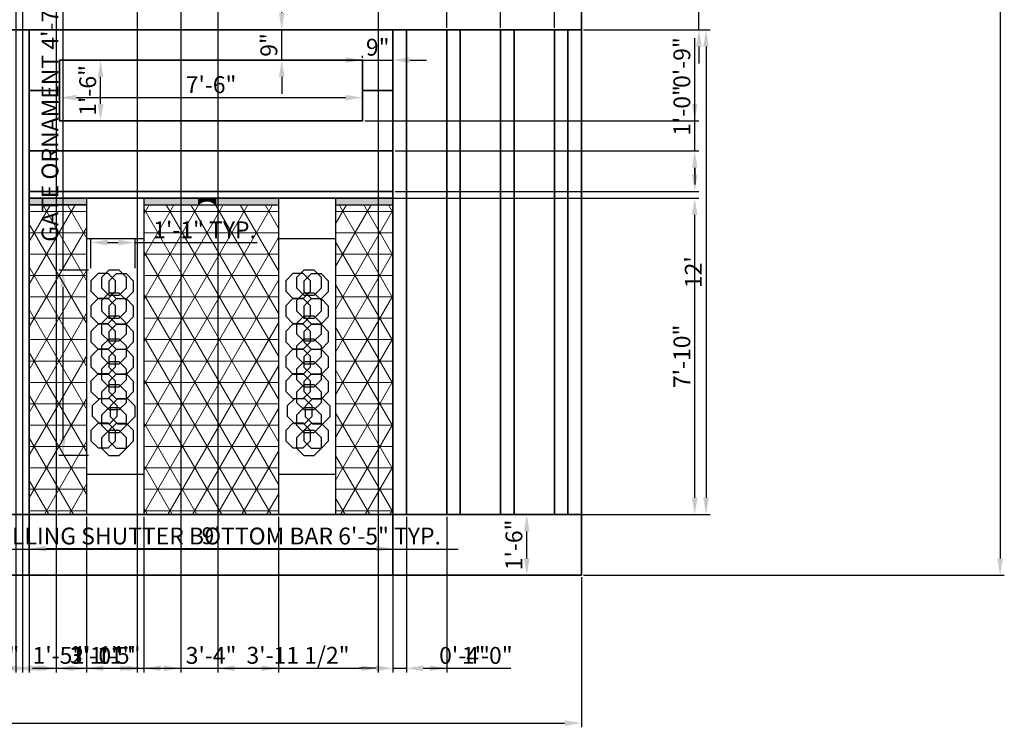
# Model space of a CAD drawing. Units: inches. Extents: x 2406 to 2953, y 1777 to 2285.
# Tile 3 of 5: x 2661 to 2953, y 1777 to 1987. Entities that reach past the tile are written whole.
import ezdxf

# ---------------------------------------------------------------- set-up
doc = ezdxf.new("R2010")
doc.units = ezdxf.units.IN
for name, color, linetype, lineweight in [('A-ANNO-DIMS', 2, 'Continuous', 18), ('A-DOOR', 3, 'Continuous', 25), ('A-ELEV', 7, 'Continuous', 35), ('A-ELEV-PATT', 253, 'Continuous', 13)]:
    doc.layers.add(name, color=color, linetype=linetype, lineweight=lineweight)
doc.styles.get("Standard").update_dxf_attribs({"font": 'arial.ttf'})
doc.dimstyles.new('ISO-25', dxfattribs={"dimtxt": 5, "dimasz": 5, "dimexe": 1.25, "dimexo": 0.625, "dimtad": 1, "dimdec": 0, "dimlunit": 3, "dimtxsty": 'Standard', "dimcen": 2.5, "dimadec": 0, "dimazin": 0, "dimtfac": 1, "dimtdec": 0, "dimtmove": 0, "dimatfit": 3, "dimfxl": 1, "dimarcsym": 0})

# ---------------------------------------------------------------- blocks, each defined once
blk = doc.blocks.new('*D1')
at = {"layer": 'A-ANNO-DIMS', "color": 0, "lineweight": -2, "transparency": 16777216}
for p, q in [((2828.46, 2242.34), (2953.44, 2242.34)), ((2952.19, 2237.34), (2952.19, 1827.34)), ((2828.46, 1822.34), (2953.44, 1822.34))]:
    blk.add_line(p, q, dxfattribs=at)
at = {"layer": 'A-ANNO-DIMS', "color": 0, "transparency": 16777216}
for points in [[(2951.35, 2237.34), (2953.02, 2237.34), (2952.19, 2242.34)], [(2951.35, 1827.34), (2953.02, 1827.34), (2952.19, 1822.34)]]:
    blk.add_solid(points, dxfattribs=at)
at = {"layer": 'Defpoints', "color": 0, "transparency": 16777216}
for p in [(2827.83, 2242.34), (2827.83, 1822.34), (2952.19, 1822.34)]:
    blk.add_point(p, dxfattribs=at)
at = {"layer": 'A-ANNO-DIMS', "color": 0, "transparency": 16777216, "insert": (2949.01, 2032.34), "char_height": 5, "attachment_point": 5, "rotation": 90}
blk.add_mtext("35'", dxfattribs=at)
blk = doc.blocks.new('*D2')
at = {"layer": 'A-ANNO-DIMS', "color": 0, "lineweight": -2, "transparency": 16777216}
for p, q in [((2443.83, 1821.72), (2443.83, 1777.16)), ((2827.83, 1821.72), (2827.83, 1777.16)), ((2448.83, 1778.41), (2822.83, 1778.41))]:
    blk.add_line(p, q, dxfattribs=at)
at = {"layer": 'A-ANNO-DIMS', "color": 0, "transparency": 16777216}
for points in [[(2448.83, 1779.24), (2448.83, 1777.58), (2443.83, 1778.41)], [(2822.83, 1779.24), (2822.83, 1777.58), (2827.83, 1778.41)]]:
    blk.add_solid(points, dxfattribs=at)
at = {"layer": 'Defpoints', "color": 0, "transparency": 16777216}
for p in [(2443.83, 1822.34), (2827.83, 1822.34), (2827.83, 1778.41)]:
    blk.add_point(p, dxfattribs=at)
at = {"layer": 'A-ANNO-DIMS', "color": 0, "transparency": 16777216, "insert": (2635.83, 1781.59), "char_height": 5, "attachment_point": 5}
blk.add_mtext("32'", dxfattribs=at)
blk = doc.blocks.new('*D3')
at = {"layer": 'A-ANNO-DIMS', "color": 0, "lineweight": -2, "transparency": 16777216}
for p, q in [((2672.83, 1957.97), (2672.83, 1965.44)), ((2762.83, 1957.97), (2762.83, 1965.44)), ((2677.83, 1964.19), (2757.83, 1964.19))]:
    blk.add_line(p, q, dxfattribs=at)
at = {"layer": 'A-ANNO-DIMS', "color": 0, "transparency": 16777216}
for points in [[(2677.83, 1965.02), (2677.83, 1963.35), (2672.83, 1964.19)], [(2757.83, 1965.02), (2757.83, 1963.35), (2762.83, 1964.19)]]:
    blk.add_solid(points, dxfattribs=at)
at = {"layer": 'Defpoints', "color": 0, "transparency": 16777216}
for p in [(2762.83, 1964.19), (2672.83, 1957.34), (2762.83, 1957.34)]:
    blk.add_point(p, dxfattribs=at)
at = {"layer": 'A-ANNO-DIMS', "color": 0, "transparency": 16777216, "insert": (2717.83, 1967.37), "char_height": 5, "attachment_point": 5}
blk.add_mtext('7\'-6"', dxfattribs=at)
blk = doc.blocks.new('*D5')
at = {"layer": 'A-ANNO-DIMS', "color": 0, "lineweight": -2, "transparency": 16777216}
for p, q in [((2828.46, 1984.34), (2866.1, 1984.34)), ((2864.85, 1979.34), (2864.85, 1845.34)), ((2828.46, 1840.34), (2866.1, 1840.34))]:
    blk.add_line(p, q, dxfattribs=at)
at = {"layer": 'A-ANNO-DIMS', "color": 0, "transparency": 16777216}
for points in [[(2864.01, 1979.34), (2865.68, 1979.34), (2864.85, 1984.34)], [(2864.01, 1845.34), (2865.68, 1845.34), (2864.85, 1840.34)]]:
    blk.add_solid(points, dxfattribs=at)
at = {"layer": 'Defpoints', "color": 0, "transparency": 16777216}
for p in [(2827.83, 1984.34), (2827.83, 1840.34), (2864.85, 1840.34)]:
    blk.add_point(p, dxfattribs=at)
at = {"layer": 'A-ANNO-DIMS', "color": 0, "transparency": 16777216, "insert": (2861.71, 1912.34), "char_height": 5, "attachment_point": 5, "rotation": 90}
blk.add_mtext("12'", dxfattribs=at)
blk = doc.blocks.new('*D16')
at = {"layer": 'A-ANNO-DIMS', "color": 0, "lineweight": -2, "transparency": 16777216}
for p, q in [((2673.46, 1975.34), (2686.26, 1975.34)), ((2685.01, 1962.34), (2685.01, 1970.34)), ((2673.46, 1957.34), (2686.26, 1957.34))]:
    blk.add_line(p, q, dxfattribs=at)
at = {"layer": 'A-ANNO-DIMS', "color": 0, "transparency": 16777216}
for points in [[(2684.18, 1970.34), (2685.85, 1970.34), (2685.01, 1975.34)], [(2684.18, 1962.34), (2685.85, 1962.34), (2685.01, 1957.34)]]:
    blk.add_solid(points, dxfattribs=at)
at = {"layer": 'Defpoints', "color": 0, "transparency": 16777216}
for p in [(2672.83, 1975.34), (2685.01, 1975.34), (2672.83, 1957.34)]:
    blk.add_point(p, dxfattribs=at)
at = {"layer": 'A-ANNO-DIMS', "color": 0, "transparency": 16777216, "insert": (2681.84, 1966.34), "char_height": 5, "attachment_point": 5, "rotation": 90}
blk.add_mtext('1\'-6"', dxfattribs=at)
blk = doc.blocks.new('*D17')
at = {"layer": 'A-ANNO-DIMS', "color": 0, "lineweight": -2, "transparency": 16777216}
for p, q in [((2663.83, 1839.72), (2663.83, 1828.98)), ((2771.83, 1839.72), (2771.83, 1828.98)), ((2668.83, 1830.23), (2766.83, 1830.23))]:
    blk.add_line(p, q, dxfattribs=at)
at = {"layer": 'A-ANNO-DIMS', "color": 0, "transparency": 16777216}
for points in [[(2668.83, 1831.07), (2668.83, 1829.4), (2663.83, 1830.23)], [(2766.83, 1831.07), (2766.83, 1829.4), (2771.83, 1830.23)]]:
    blk.add_solid(points, dxfattribs=at)
at = {"layer": 'Defpoints', "color": 0, "transparency": 16777216}
for p in [(2663.83, 1840.34), (2771.83, 1840.34), (2771.83, 1830.23)]:
    blk.add_point(p, dxfattribs=at)
at = {"layer": 'A-ANNO-DIMS', "color": 0, "transparency": 16777216, "insert": (2717.83, 1833.41), "char_height": 5, "attachment_point": 5}
blk.add_mtext("9'", dxfattribs=at)
blk = doc.blocks.new('*D18')
at = {"layer": 'A-ANNO-DIMS', "color": 0, "lineweight": -2, "transparency": 16777216}
for p, q in [((2827.21, 1840.34), (2810.34, 1840.34)), ((2811.59, 1827.34), (2811.59, 1835.34)), ((2827.21, 1822.34), (2810.34, 1822.34))]:
    blk.add_line(p, q, dxfattribs=at)
at = {"layer": 'A-ANNO-DIMS', "color": 0, "transparency": 16777216}
for points in [[(2810.76, 1835.34), (2812.43, 1835.34), (2811.59, 1840.34)], [(2810.76, 1827.34), (2812.43, 1827.34), (2811.59, 1822.34)]]:
    blk.add_solid(points, dxfattribs=at)
at = {"layer": 'Defpoints', "color": 0, "transparency": 16777216}
for p in [(2811.59, 1840.34), (2827.83, 1840.34), (2827.83, 1822.34)]:
    blk.add_point(p, dxfattribs=at)
at = {"layer": 'A-ANNO-DIMS', "color": 0, "transparency": 16777216, "insert": (2808.42, 1831.34), "char_height": 5, "attachment_point": 5, "rotation": 90}
blk.add_mtext('1\'-6"', dxfattribs=at)
blk = doc.blocks.new('*D19')
at = {"layer": 'A-ANNO-DIMS', "color": 0, "lineweight": -2, "transparency": 16777216}
for p, q in [((2862.73, 1995.34), (2862.73, 2007.37)), ((2828.46, 1990.34), (2863.98, 1990.34)), ((2862.73, 1984.34), (2862.73, 1990.34)), ((2828.46, 1984.34), (2863.98, 1984.34)), ((2862.73, 1979.34), (2862.73, 1974.34))]:
    blk.add_line(p, q, dxfattribs=at)
at = {"layer": 'A-ANNO-DIMS', "color": 0, "transparency": 16777216}
for points in [[(2861.89, 1995.34), (2863.56, 1995.34), (2862.73, 1990.34)], [(2861.89, 1979.34), (2863.56, 1979.34), (2862.73, 1984.34)]]:
    blk.add_solid(points, dxfattribs=at)
at = {"layer": 'Defpoints', "color": 0, "transparency": 16777216}
for p in [(2827.83, 1990.34), (2862.73, 1990.34), (2827.83, 1984.34)]:
    blk.add_point(p, dxfattribs=at)
at = {"layer": 'A-ANNO-DIMS', "color": 0, "transparency": 16777216, "insert": (2859.55, 2003.85), "char_height": 5, "attachment_point": 5, "rotation": 90}
blk.add_mtext('6"', dxfattribs=at)
blk = doc.blocks.new('*D31')
at = {"layer": 'A-ANNO-DIMS', "color": 0, "lineweight": -2, "transparency": 16777216}
for p, q in [((2757.83, 1975.34), (2752.83, 1975.34)), ((2762.83, 1975.97), (2762.83, 1976.59)), ((2762.83, 1975.34), (2771.83, 1975.34)), ((2771.83, 1975.97), (2771.83, 1976.59)), ((2776.83, 1975.34), (2781.83, 1975.34))]:
    blk.add_line(p, q, dxfattribs=at)
at = {"layer": 'A-ANNO-DIMS', "color": 0, "transparency": 16777216}
for points in [[(2757.83, 1976.17), (2757.83, 1974.51), (2762.83, 1975.34)], [(2776.83, 1976.17), (2776.83, 1974.51), (2771.83, 1975.34)]]:
    blk.add_solid(points, dxfattribs=at)
at = {"layer": 'Defpoints', "color": 0, "transparency": 16777216}
for p in [(2762.83, 1975.34), (2771.83, 1975.34), (2771.83, 1975.34)]:
    blk.add_point(p, dxfattribs=at)
at = {"layer": 'A-ANNO-DIMS', "color": 0, "transparency": 16777216, "insert": (2767.33, 1978.52), "char_height": 5, "attachment_point": 5}
blk.add_mtext('9"', dxfattribs=at)
blk = doc.blocks.new('*D32')
at = {"layer": 'A-ANNO-DIMS', "color": 0, "lineweight": -2, "transparency": 16777216}
for p, q in [((2738.81, 1989.34), (2738.81, 1994.34)), ((2748.35, 1984.34), (2737.56, 1984.34)), ((2738.81, 1975.34), (2738.81, 1984.34)), ((2748.35, 1975.34), (2737.56, 1975.34)), ((2738.81, 1970.34), (2738.81, 1965.34))]:
    blk.add_line(p, q, dxfattribs=at)
at = {"layer": 'A-ANNO-DIMS', "color": 0, "transparency": 16777216}
for points in [[(2737.98, 1989.34), (2739.65, 1989.34), (2738.81, 1984.34)], [(2737.98, 1970.34), (2739.65, 1970.34), (2738.81, 1975.34)]]:
    blk.add_solid(points, dxfattribs=at)
at = {"layer": 'Defpoints', "color": 0, "transparency": 16777216}
for p in [(2738.81, 1984.34), (2748.98, 1984.34), (2748.98, 1975.34)]:
    blk.add_point(p, dxfattribs=at)
at = {"layer": 'A-ANNO-DIMS', "color": 0, "transparency": 16777216, "insert": (2735.64, 1979.84), "char_height": 5, "attachment_point": 5, "rotation": 90}
blk.add_mtext('9"', dxfattribs=at)
blk = doc.blocks.new('GATE-ORNAMENT')
for points in [[(7.37, 51.86), (5.21, 54.02), (2.16, 54.02), (0, 51.86), (0, 48.81), (2.16, 46.65), (5.21, 46.65), (7.37, 48.81)], [(10.58, 52.83), (8.42, 54.99), (5.37, 54.99), (3.21, 52.83), (3.21, 49.78), (5.37, 47.62), (8.42, 47.62), (10.58, 49.78)], [(12.73, 51.79), (10.58, 53.95), (7.52, 53.95), (5.37, 51.79), (5.37, 48.74), (7.52, 46.58), (10.58, 46.58), (12.73, 48.74)], [(10.58, 46.03), (8.42, 48.18), (5.37, 48.18), (3.21, 46.03), (3.21, 42.97), (5.37, 40.82), (8.42, 40.82), (10.58, 42.97)], [(7.37, 44.42), (5.21, 46.58), (2.16, 46.58), (0, 44.42), (0, 41.37), (2.16, 39.21), (5.21, 39.21), (7.37, 41.37)], [(12.73, 44.35), (10.58, 46.5), (7.52, 46.5), (5.37, 44.35), (5.37, 41.29), (7.52, 39.14), (10.58, 39.14), (12.73, 41.29)], [(10.58, 39.22), (8.42, 41.38), (5.37, 41.38), (3.21, 39.22), (3.21, 36.17), (5.37, 34.01), (8.42, 34.01), (10.58, 36.17)], [(7.37, 36.82), (5.21, 38.98), (2.16, 38.98), (0, 36.82), (0, 33.77), (2.16, 31.61), (5.21, 31.61), (7.37, 33.77)], [(12.73, 36.75), (10.58, 38.91), (7.52, 38.91), (5.37, 36.75), (5.37, 33.7), (7.52, 31.54), (10.58, 31.54), (12.73, 33.7)], [(10.58, 32.42), (8.42, 34.58), (5.37, 34.58), (3.21, 32.42), (3.21, 29.37), (5.37, 27.21), (8.42, 27.21), (10.58, 29.37)], [(7.37, 29.4), (5.21, 31.56), (2.16, 31.56), (0, 29.4), (0, 26.35), (2.16, 24.19), (5.21, 24.19), (7.37, 26.35)], [(12.73, 29.33), (10.58, 31.48), (7.52, 31.48), (5.37, 29.33), (5.37, 26.27), (7.52, 24.12), (10.58, 24.12), (12.73, 26.27)], [(10.58, 25.62), (8.42, 27.78), (5.37, 27.78), (3.21, 25.62), (3.21, 22.57), (5.37, 20.41), (8.42, 20.41), (10.58, 22.57)], [(7.37, 22.08), (5.21, 24.24), (2.16, 24.24), (0, 22.08), (0, 19.03), (2.16, 16.87), (5.21, 16.87), (7.37, 19.03)], [(12.73, 22), (10.58, 24.16), (7.52, 24.16), (5.37, 22), (5.37, 18.95), (7.52, 16.8), (10.58, 16.8), (12.73, 18.95)], [(10.58, 18.81), (8.42, 20.97), (5.37, 20.97), (3.21, 18.81), (3.21, 15.76), (5.37, 13.61), (8.42, 13.61), (10.58, 15.76)], [(7.81, 14.69), (5.66, 16.85), (2.61, 16.85), (0.45, 14.69), (0.45, 11.64), (2.61, 9.48), (5.66, 9.48), (7.81, 11.64)], [(13.18, 14.62), (11.02, 16.77), (7.97, 16.77), (5.81, 14.62), (5.81, 11.57), (7.97, 9.41), (11.02, 9.41), (13.18, 11.57)], [(10.58, 12.01), (8.42, 14.17), (5.37, 14.17), (3.21, 12.01), (3.21, 8.96), (5.37, 6.8), (8.42, 6.8), (10.58, 8.96)], [(7.37, 7.44), (5.21, 9.6), (2.16, 9.6), (0, 7.44), (0, 4.39), (2.16, 2.23), (5.21, 2.23), (7.37, 4.39)], [(12.73, 7.37), (10.58, 9.52), (7.52, 9.52), (5.37, 7.37), (5.37, 4.32), (7.52, 2.16), (10.58, 2.16), (12.73, 4.32)], [(10.58, 5.21), (8.42, 7.37), (5.37, 7.37), (3.21, 5.21), (3.21, 2.16), (5.37, 0), (8.42, 0), (10.58, 2.16)]]:
    blk.add_lwpolyline(points, close=True)
blk = doc.blocks.new('*D43')
at = {"layer": 'A-ANNO-DIMS', "color": 0, "lineweight": -2, "transparency": 16777216}
for p, q in [((2562.31, 1841.02), (2562.31, 1828.87)), ((2639.14, 1841.02), (2639.14, 1828.87)), ((2567.31, 1830.12), (2634.14, 1830.12)), ((2639.14, 1830.12), (2791.26, 1830.12))]:
    blk.add_line(p, q, dxfattribs=at)
at = {"layer": 'A-ANNO-DIMS', "color": 0, "transparency": 16777216}
for points in [[(2567.31, 1830.96), (2567.31, 1829.29), (2562.31, 1830.12)], [(2634.14, 1830.96), (2634.14, 1829.29), (2639.14, 1830.12)]]:
    blk.add_solid(points, dxfattribs=at)
at = {"layer": 'Defpoints', "color": 0, "transparency": 16777216}
for p in [(2562.31, 1841.65), (2639.14, 1841.65), (2639.14, 1830.12)]:
    blk.add_point(p, dxfattribs=at)
at = {"layer": 'A-ANNO-DIMS', "color": 0, "transparency": 16777216, "insert": (2717.7, 1833.33), "char_height": 5, "attachment_point": 5}
blk.add_mtext('ROLLING SHUTTER BOTTOM BAR 6\'-5" TYP.', dxfattribs=at)
blk = doc.blocks.new('*D45')
at = {"layer": 'A-ANNO-DIMS', "color": 0, "lineweight": -2, "transparency": 16777216}
for p, q in [((2673.85, 1912.9), (2673.85, 2012.41)), ((2681.47, 1912.9), (2672.6, 1912.9)), ((2673.85, 1862.91), (2673.85, 1907.9)), ((2681.47, 1857.91), (2672.6, 1857.91))]:
    blk.add_line(p, q, dxfattribs=at)
at = {"layer": 'A-ANNO-DIMS', "color": 0, "transparency": 16777216}
for points in [[(2673.01, 1907.9), (2674.68, 1907.9), (2673.85, 1912.9)], [(2673.01, 1862.91), (2674.68, 1862.91), (2673.85, 1857.91)]]:
    blk.add_solid(points, dxfattribs=at)
at = {"layer": 'Defpoints', "color": 0, "transparency": 16777216}
for p in [(2673.85, 1912.9), (2682.1, 1912.9), (2682.1, 1857.91)]:
    blk.add_point(p, dxfattribs=at)
at = {"layer": 'A-ANNO-DIMS', "color": 0, "transparency": 16777216, "insert": (2670.64, 1965.16), "char_height": 5, "attachment_point": 5, "rotation": 90}
blk.add_mtext('GATE ORNAMENT 4\'-7" TYP.', dxfattribs=at)
blk = doc.blocks.new('*D46')
at = {"layer": 'A-ANNO-DIMS', "color": 0, "lineweight": -2, "transparency": 16777216}
for p, q in [((2682.1, 1913.52), (2682.1, 1922.4)), ((2695.28, 1913.52), (2695.28, 1922.4)), ((2687.1, 1921.15), (2690.28, 1921.15)), ((2695.28, 1921.15), (2731.53, 1921.15))]:
    blk.add_line(p, q, dxfattribs=at)
at = {"layer": 'A-ANNO-DIMS', "color": 0, "transparency": 16777216}
for points in [[(2687.1, 1921.98), (2687.1, 1920.31), (2682.1, 1921.15)], [(2690.28, 1921.98), (2690.28, 1920.31), (2695.28, 1921.15)]]:
    blk.add_solid(points, dxfattribs=at)
at = {"layer": 'Defpoints', "color": 0, "transparency": 16777216}
for p in [(2695.28, 1921.15), (2682.1, 1912.9), (2695.28, 1912.9)]:
    blk.add_point(p, dxfattribs=at)
at = {"layer": 'A-ANNO-DIMS', "color": 0, "transparency": 16777216, "insert": (2715.9, 1924.28), "char_height": 5, "attachment_point": 5}
blk.add_mtext('1\'-1" TYP.', dxfattribs=at)
blk = doc.blocks.new('*D48')
at = {"layer": 'A-ANNO-DIMS', "color": 0, "lineweight": -2, "transparency": 16777216}
for p, q in [((2642.83, 1839.72), (2642.83, 1793.44)), ((2663.83, 1839.72), (2663.83, 1793.44)), ((2647.83, 1794.69), (2658.83, 1794.69))]:
    blk.add_line(p, q, dxfattribs=at)
at = {"layer": 'A-ANNO-DIMS', "color": 0, "transparency": 16777216}
for points in [[(2647.83, 1795.52), (2647.83, 1793.86), (2642.83, 1794.69)], [(2658.83, 1795.52), (2658.83, 1793.86), (2663.83, 1794.69)]]:
    blk.add_solid(points, dxfattribs=at)
at = {"layer": 'Defpoints', "color": 0, "transparency": 16777216}
for p in [(2642.83, 1840.34), (2663.83, 1840.34), (2663.83, 1794.69)]:
    blk.add_point(p, dxfattribs=at)
at = {"layer": 'A-ANNO-DIMS', "color": 0, "transparency": 16777216, "insert": (2653.33, 1797.87), "char_height": 5, "attachment_point": 5}
blk.add_mtext('1\'-9"', dxfattribs=at)
blk = doc.blocks.new('*D49')
at = {"layer": 'A-ANNO-DIMS', "color": 0, "lineweight": -2, "transparency": 16777216}
for p, q in [((2771.83, 1839.72), (2771.83, 1793.44)), ((2775.83, 1839.72), (2775.83, 1793.44)), ((2766.83, 1794.69), (2761.83, 1794.69)), ((2771.83, 1794.69), (2775.83, 1794.69)), ((2780.83, 1794.69), (2800.37, 1794.69))]:
    blk.add_line(p, q, dxfattribs=at)
at = {"layer": 'A-ANNO-DIMS', "color": 0, "transparency": 16777216}
for points in [[(2766.83, 1795.52), (2766.83, 1793.86), (2771.83, 1794.69)], [(2780.83, 1795.52), (2780.83, 1793.86), (2775.83, 1794.69)]]:
    blk.add_solid(points, dxfattribs=at)
at = {"layer": 'Defpoints', "color": 0, "transparency": 16777216}
for p in [(2771.83, 1840.34), (2775.83, 1840.34), (2775.83, 1794.69)]:
    blk.add_point(p, dxfattribs=at)
at = {"layer": 'A-ANNO-DIMS', "color": 0, "transparency": 16777216, "insert": (2793.1, 1797.87), "char_height": 5, "attachment_point": 5}
blk.add_mtext('0\'-4"', dxfattribs=at)
blk = doc.blocks.new('*D50')
at = {"layer": 'A-ANNO-DIMS', "color": 0, "lineweight": -2, "transparency": 16777216}
for p, q in [((2775.83, 1839.72), (2775.83, 1793.44)), ((2787.83, 1839.72), (2787.83, 1793.44)), ((2780.83, 1794.69), (2782.83, 1794.69)), ((2787.83, 1794.69), (2806.9, 1794.69))]:
    blk.add_line(p, q, dxfattribs=at)
at = {"layer": 'A-ANNO-DIMS', "color": 0, "transparency": 16777216}
for points in [[(2780.83, 1795.52), (2780.83, 1793.86), (2775.83, 1794.69)], [(2782.83, 1795.52), (2782.83, 1793.86), (2787.83, 1794.69)]]:
    blk.add_solid(points, dxfattribs=at)
at = {"layer": 'Defpoints', "color": 0, "transparency": 16777216}
for p in [(2775.83, 1840.34), (2787.83, 1840.34), (2787.83, 1794.69)]:
    blk.add_point(p, dxfattribs=at)
at = {"layer": 'A-ANNO-DIMS', "color": 0, "transparency": 16777216, "insert": (2799.87, 1797.87), "char_height": 5, "attachment_point": 5}
blk.add_mtext('1\'-0"', dxfattribs=at)
blk = doc.blocks.new('*D51')
at = {"layer": 'A-ANNO-DIMS', "color": 0, "lineweight": -2, "transparency": 16777216}
for p, q in [((2787.83, 1984.97), (2787.83, 2275.24)), ((2792.83, 2273.99), (2798.83, 2273.99)), ((2803.83, 1984.97), (2803.83, 2275.24))]:
    blk.add_line(p, q, dxfattribs=at)
at = {"layer": 'A-ANNO-DIMS', "color": 0, "transparency": 16777216}
for points in [[(2792.83, 2274.82), (2792.83, 2273.16), (2787.83, 2273.99)], [(2798.83, 2274.82), (2798.83, 2273.16), (2803.83, 2273.99)]]:
    blk.add_solid(points, dxfattribs=at)
at = {"layer": 'Defpoints', "color": 0, "transparency": 16777216}
for p in [(2803.83, 2273.99), (2787.83, 1984.34), (2803.83, 1984.34)]:
    blk.add_point(p, dxfattribs=at)
at = {"layer": 'A-ANNO-DIMS', "color": 0, "transparency": 16777216, "insert": (2795.83, 2277.13), "char_height": 5, "attachment_point": 5}
blk.add_mtext('1\'-4"', dxfattribs=at)
blk = doc.blocks.new('*D52')
at = {"layer": 'A-ANNO-DIMS', "color": 0, "lineweight": -2, "transparency": 16777216}
for p, q in [((2803.83, 1984.97), (2803.83, 2275.24)), ((2808.83, 2273.99), (2814.83, 2273.99)), ((2819.83, 1984.97), (2819.83, 2275.24))]:
    blk.add_line(p, q, dxfattribs=at)
at = {"layer": 'A-ANNO-DIMS', "color": 0, "transparency": 16777216}
for points in [[(2808.83, 2274.82), (2808.83, 2273.16), (2803.83, 2273.99)], [(2814.83, 2274.82), (2814.83, 2273.16), (2819.83, 2273.99)]]:
    blk.add_solid(points, dxfattribs=at)
at = {"layer": 'Defpoints', "color": 0, "transparency": 16777216}
for p in [(2819.83, 2273.99), (2803.83, 1984.34), (2819.83, 1984.34)]:
    blk.add_point(p, dxfattribs=at)
at = {"layer": 'A-ANNO-DIMS', "color": 0, "transparency": 16777216, "insert": (2811.83, 2277.13), "char_height": 5, "attachment_point": 5}
blk.add_mtext('1\'-4"', dxfattribs=at)
blk = doc.blocks.new('*D53')
at = {"layer": 'A-ANNO-DIMS', "color": 0, "lineweight": -2, "transparency": 16777216}
for p, q in [((2814.83, 2273.99), (2809.83, 2273.99)), ((2819.83, 1984.97), (2819.83, 2275.24)), ((2819.83, 2273.99), (2827.83, 2273.99)), ((2827.83, 1984.97), (2827.83, 2275.24)), ((2832.83, 2273.99), (2852.37, 2273.99))]:
    blk.add_line(p, q, dxfattribs=at)
at = {"layer": 'A-ANNO-DIMS', "color": 0, "transparency": 16777216}
for points in [[(2814.83, 2274.82), (2814.83, 2273.16), (2819.83, 2273.99)], [(2832.83, 2274.82), (2832.83, 2273.16), (2827.83, 2273.99)]]:
    blk.add_solid(points, dxfattribs=at)
at = {"layer": 'Defpoints', "color": 0, "transparency": 16777216}
for p in [(2827.83, 2273.99), (2819.83, 1984.34), (2827.83, 1984.34)]:
    blk.add_point(p, dxfattribs=at)
at = {"layer": 'A-ANNO-DIMS', "color": 0, "transparency": 16777216, "insert": (2845.1, 2277.17), "char_height": 5, "attachment_point": 5}
blk.add_mtext('0\'-8"', dxfattribs=at)
blk = doc.blocks.new('*D56')
at = {"layer": 'A-ANNO-DIMS', "color": 0, "lineweight": -2, "transparency": 16777216}
for p, q in [((2664.46, 1934.34), (2862.73, 1934.34)), ((2861.48, 1845.34), (2861.48, 1929.34)), ((2664.46, 1840.34), (2862.73, 1840.34))]:
    blk.add_line(p, q, dxfattribs=at)
at = {"layer": 'A-ANNO-DIMS', "color": 0, "transparency": 16777216}
for points in [[(2860.65, 1929.34), (2862.32, 1929.34), (2861.48, 1934.34)], [(2860.65, 1845.34), (2862.32, 1845.34), (2861.48, 1840.34)]]:
    blk.add_solid(points, dxfattribs=at)
at = {"layer": 'Defpoints', "color": 0, "transparency": 16777216}
for p in [(2663.83, 1934.34), (2861.48, 1934.34), (2663.83, 1840.34)]:
    blk.add_point(p, dxfattribs=at)
at = {"layer": 'A-ANNO-DIMS', "color": 0, "transparency": 16777216, "insert": (2858.31, 1887.34), "char_height": 5, "attachment_point": 5, "rotation": 90}
blk.add_mtext('7\'-10"', dxfattribs=at)
blk = doc.blocks.new('*D57')
at = {"layer": 'A-ANNO-DIMS', "color": 0, "lineweight": -2, "transparency": 16777216}
for p, q in [((2861.48, 1948.34), (2861.48, 1967.41)), ((2772.46, 1948.34), (2862.73, 1948.34)), ((2861.48, 1941.34), (2861.48, 1943.34)), ((2772.46, 1936.34), (2862.73, 1936.34))]:
    blk.add_line(p, q, dxfattribs=at)
at = {"layer": 'A-ANNO-DIMS', "color": 0, "transparency": 16777216}
for points in [[(2860.65, 1943.34), (2862.32, 1943.34), (2861.48, 1948.34)], [(2860.65, 1941.34), (2862.32, 1941.34), (2861.48, 1936.34)]]:
    blk.add_solid(points, dxfattribs=at)
at = {"layer": 'Defpoints', "color": 0, "transparency": 16777216}
for p in [(2771.83, 1948.34), (2861.48, 1948.34), (2771.83, 1936.34)]:
    blk.add_point(p, dxfattribs=at)
at = {"layer": 'A-ANNO-DIMS', "color": 0, "transparency": 16777216, "insert": (2858.31, 1960.38), "char_height": 5, "attachment_point": 5, "rotation": 90}
blk.add_mtext('1\'-0"', dxfattribs=at)
blk = doc.blocks.new('*D58')
at = {"layer": 'A-ANNO-DIMS', "color": 0, "lineweight": -2, "transparency": 16777216}
for p, q in [((2861.48, 1962.34), (2861.48, 1981.88)), ((2763.46, 1957.34), (2862.73, 1957.34)), ((2861.48, 1948.34), (2861.48, 1957.34)), ((2772.46, 1948.34), (2862.73, 1948.34)), ((2861.48, 1943.34), (2861.48, 1938.34))]:
    blk.add_line(p, q, dxfattribs=at)
at = {"layer": 'A-ANNO-DIMS', "color": 0, "transparency": 16777216}
for points in [[(2860.65, 1962.34), (2862.32, 1962.34), (2861.48, 1957.34)], [(2860.65, 1943.34), (2862.32, 1943.34), (2861.48, 1948.34)]]:
    blk.add_solid(points, dxfattribs=at)
at = {"layer": 'Defpoints', "color": 0, "transparency": 16777216}
for p in [(2762.83, 1957.34), (2861.48, 1957.34), (2771.83, 1948.34)]:
    blk.add_point(p, dxfattribs=at)
at = {"layer": 'A-ANNO-DIMS', "color": 0, "transparency": 16777216, "insert": (2858.31, 1974.61), "char_height": 5, "attachment_point": 5, "rotation": 90}
blk.add_mtext('0\'-9"', dxfattribs=at)
blk = doc.blocks.new('*D59')
at = {"layer": 'A-ANNO-DIMS', "color": 0, "lineweight": -2, "transparency": 16777216}
for p, q in [((2663.83, 1839.72), (2663.83, 1793.44)), ((2680.83, 1839.72), (2680.83, 1793.44)), ((2668.83, 1794.69), (2675.83, 1794.69))]:
    blk.add_line(p, q, dxfattribs=at)
at = {"layer": 'A-ANNO-DIMS', "color": 0, "transparency": 16777216}
for points in [[(2668.83, 1795.52), (2668.83, 1793.86), (2663.83, 1794.69)], [(2675.83, 1795.52), (2675.83, 1793.86), (2680.83, 1794.69)]]:
    blk.add_solid(points, dxfattribs=at)
at = {"layer": 'Defpoints', "color": 0, "transparency": 16777216}
for p in [(2663.83, 1840.34), (2680.83, 1840.34), (2680.83, 1794.69)]:
    blk.add_point(p, dxfattribs=at)
at = {"layer": 'A-ANNO-DIMS', "color": 0, "transparency": 16777216, "insert": (2672.33, 1797.87), "char_height": 5, "attachment_point": 5}
blk.add_mtext('1\'-5"', dxfattribs=at)
blk = doc.blocks.new('*D60')
at = {"layer": 'A-ANNO-DIMS', "color": 0, "lineweight": -2, "transparency": 16777216}
for p, q in [((2680.83, 1839.72), (2680.83, 1793.44)), ((2697.83, 1839.72), (2697.83, 1793.44)), ((2685.83, 1794.69), (2692.83, 1794.69))]:
    blk.add_line(p, q, dxfattribs=at)
at = {"layer": 'A-ANNO-DIMS', "color": 0, "transparency": 16777216}
for points in [[(2685.83, 1795.52), (2685.83, 1793.86), (2680.83, 1794.69)], [(2692.83, 1795.52), (2692.83, 1793.86), (2697.83, 1794.69)]]:
    blk.add_solid(points, dxfattribs=at)
at = {"layer": 'Defpoints', "color": 0, "transparency": 16777216}
for p in [(2680.83, 1840.34), (2697.83, 1840.34), (2697.83, 1794.69)]:
    blk.add_point(p, dxfattribs=at)
at = {"layer": 'A-ANNO-DIMS', "color": 0, "transparency": 16777216, "insert": (2689.33, 1797.87), "char_height": 5, "attachment_point": 5}
blk.add_mtext('1\'-5"', dxfattribs=at)
blk = doc.blocks.new('*D61')
at = {"layer": 'A-ANNO-DIMS', "color": 0, "lineweight": -2, "transparency": 16777216}
for p, q in [((2697.83, 1839.72), (2697.83, 1793.44)), ((2737.83, 1839.72), (2737.83, 1793.44)), ((2702.83, 1794.69), (2732.83, 1794.69))]:
    blk.add_line(p, q, dxfattribs=at)
at = {"layer": 'A-ANNO-DIMS', "color": 0, "transparency": 16777216}
for points in [[(2702.83, 1795.52), (2702.83, 1793.86), (2697.83, 1794.69)], [(2732.83, 1795.52), (2732.83, 1793.86), (2737.83, 1794.69)]]:
    blk.add_solid(points, dxfattribs=at)
at = {"layer": 'Defpoints', "color": 0, "transparency": 16777216}
for p in [(2697.83, 1840.34), (2737.83, 1840.34), (2737.83, 1794.69)]:
    blk.add_point(p, dxfattribs=at)
at = {"layer": 'A-ANNO-DIMS', "color": 0, "transparency": 16777216, "insert": (2717.83, 1797.87), "char_height": 5, "attachment_point": 5}
blk.add_mtext('3\'-4"', dxfattribs=at)
blk = doc.blocks.new('*D64')
at = {"layer": 'A-ANNO-DIMS', "color": 0, "lineweight": -2, "transparency": 16777216}
for p, q in [((2659.83, 2103.72), (2659.83, 1793.44)), ((2671.83, 2089.72), (2671.83, 1793.44)), ((2664.83, 1794.69), (2666.83, 1794.69)), ((2671.83, 1794.69), (2690.9, 1794.69))]:
    blk.add_line(p, q, dxfattribs=at)
at = {"layer": 'A-ANNO-DIMS', "color": 0, "transparency": 16777216}
for points in [[(2664.83, 1795.52), (2664.83, 1793.86), (2659.83, 1794.69)], [(2666.83, 1795.52), (2666.83, 1793.86), (2671.83, 1794.69)]]:
    blk.add_solid(points, dxfattribs=at)
at = {"layer": 'Defpoints', "color": 0, "transparency": 16777216}
for p in [(2659.83, 2104.34), (2671.83, 2090.34), (2671.83, 1794.69)]:
    blk.add_point(p, dxfattribs=at)
at = {"layer": 'A-ANNO-DIMS', "color": 0, "transparency": 16777216, "insert": (2683.87, 1797.87), "char_height": 5, "attachment_point": 5}
blk.add_mtext('1\'-0"', dxfattribs=at)
blk = doc.blocks.new('*D65')
at = {"layer": 'A-ANNO-DIMS', "color": 0, "lineweight": -2, "transparency": 16777216}
for p, q in [((2671.83, 2089.72), (2671.83, 1793.44)), ((2695.83, 2089.72), (2695.83, 1793.44)), ((2676.83, 1794.69), (2690.83, 1794.69))]:
    blk.add_line(p, q, dxfattribs=at)
at = {"layer": 'A-ANNO-DIMS', "color": 0, "transparency": 16777216}
for points in [[(2676.83, 1795.52), (2676.83, 1793.86), (2671.83, 1794.69)], [(2690.83, 1795.52), (2690.83, 1793.86), (2695.83, 1794.69)]]:
    blk.add_solid(points, dxfattribs=at)
at = {"layer": 'Defpoints', "color": 0, "transparency": 16777216}
for p in [(2671.83, 2090.34), (2695.83, 2090.34), (2695.83, 1794.69)]:
    blk.add_point(p, dxfattribs=at)
at = {"layer": 'A-ANNO-DIMS', "color": 0, "transparency": 16777216, "insert": (2683.83, 1797.87), "char_height": 5, "attachment_point": 5}
blk.add_mtext('2\'-0"', dxfattribs=at)
blk = doc.blocks.new('*D67')
at = {"layer": 'A-ANNO-DIMS', "color": 0, "lineweight": -2, "transparency": 16777216}
for p, q in [((2719.83, 2007.72), (2719.83, 1793.44)), ((2767.46, 2007.72), (2767.46, 1793.44)), ((2724.83, 1794.69), (2762.46, 1794.69))]:
    blk.add_line(p, q, dxfattribs=at)
at = {"layer": 'A-ANNO-DIMS', "color": 0, "transparency": 16777216}
for points in [[(2724.83, 1795.52), (2724.83, 1793.86), (2719.83, 1794.69)], [(2762.46, 1795.52), (2762.46, 1793.86), (2767.46, 1794.69)]]:
    blk.add_solid(points, dxfattribs=at)
at = {"layer": 'Defpoints', "color": 0, "transparency": 16777216}
for p in [(2719.83, 2008.34), (2767.46, 2008.34), (2767.46, 1794.69)]:
    blk.add_point(p, dxfattribs=at)
at = {"layer": 'A-ANNO-DIMS', "color": 0, "transparency": 16777216, "insert": (2743.65, 1797.9), "char_height": 5, "attachment_point": 5}
blk.add_mtext('3\'-11 1/2"', dxfattribs=at)
blk = doc.blocks.new('*D82')
at = {"layer": 'A-ANNO-DIMS', "color": 0, "lineweight": -2, "transparency": 16777216}
for p, q in [((2661.83, 2155.72), (2661.83, 1793.44)), ((2708.83, 2155.72), (2708.83, 1793.44)), ((2666.83, 1794.69), (2703.83, 1794.69))]:
    blk.add_line(p, q, dxfattribs=at)
at = {"layer": 'A-ANNO-DIMS', "color": 0, "transparency": 16777216}
for points in [[(2666.83, 1795.52), (2666.83, 1793.86), (2661.83, 1794.69)], [(2703.83, 1795.52), (2703.83, 1793.86), (2708.83, 1794.69)]]:
    blk.add_solid(points, dxfattribs=at)
at = {"layer": 'Defpoints', "color": 0, "transparency": 16777216}
for p in [(2661.83, 2156.34), (2708.83, 2156.34), (2708.83, 1794.69)]:
    blk.add_point(p, dxfattribs=at)
at = {"layer": 'A-ANNO-DIMS', "color": 0, "transparency": 16777216, "insert": (2685.33, 1797.87), "char_height": 5, "attachment_point": 5}
blk.add_mtext('3\'-11"', dxfattribs=at)

msp = doc.modelspace()

# ---------------------------------------------------------------- hatches: boundary and pattern name
at = {"layer": 'A-ELEV-PATT'}
h = msp.add_hatch(color=256, dxfattribs=at)
h.dxf.hatch_style = 1
h.paths.add_polyline_path([(2680.83, 1932.34), (2680.83, 1934.34), (2663.83, 1934.34), (2663.83, 1932.34)])
h = msp.add_hatch(color=256, dxfattribs=at)
h.dxf.hatch_style = 1
h.paths.add_polyline_path([(2697.83, 1934.34), (2697.83, 1932.34), (2714.05, 1932.34), (2714.05, 1934.34)])
h = msp.add_hatch(dxfattribs=at)
h.set_pattern_fill('BRICK', color=256, scale=0.5)
h.set_pattern_definition([(0, (0, 0), (0, 0.125), []), (90, (0, 0), (-0.25, 0), [0.125, -0.125]), (90, (0.125, 0), (-0.25, 0), [-0.125, 0.125])])
h.paths.add_polyline_path([(2719.19, 1932.34), (2719.19, 1934.34), (2714.05, 1934.34), (2714.05, 1932.34, -0.437188)])
h = msp.add_hatch(color=256, dxfattribs=at)
h.dxf.hatch_style = 1
h.paths.add_polyline_path([(2737.83, 1932.34), (2737.83, 1934.34), (2719.19, 1934.34), (2719.19, 1932.34)])
h = msp.add_hatch(color=256, dxfattribs=at)
h.dxf.hatch_style = 1
h.paths.add_polyline_path([(2771.83, 1932.34), (2771.83, 1934.34), (2754.83, 1934.34), (2754.83, 1932.34)])
h = msp.add_hatch(dxfattribs=at)
h.set_pattern_fill('NET3', color=256, scale=2)
h.paths.add_polyline_path([(2680.83, 1932.34), (2663.83, 1932.34), (2663.83, 1840.34), (2680.83, 1840.34)])
h.paths.add_polyline_path([(2737.83, 1932.34), (2697.83, 1932.34), (2697.83, 1840.34), (2737.83, 1840.34)])
h.paths.add_polyline_path([(2771.83, 1932.34), (2754.83, 1932.34), (2754.83, 1840.34), (2771.83, 1840.34)])

# ---------------------------------------------------------------- linework, layer by layer
at = {"layer": 'A-DOOR'}
for p, q in [((2714.05, 1936.34), (2719.19, 1936.34)), ((2680.83, 1934.34), (2680.83, 1840.34)), ((2697.83, 1934.34), (2697.83, 1840.34)), ((2719.19, 1934.34), (2714.05, 1934.34)), ((2714.05, 1934.34), (2714.05, 1932.34)), ((2719.19, 1934.34), (2719.19, 1932.34)), ((2737.83, 1934.34), (2737.83, 1840.34)), ((2754.83, 1934.34), (2754.83, 1840.34)), ((2697.83, 1932.34), (2737.83, 1932.34)), ((2754.83, 1932.34), (2771.83, 1932.34)), ((2680.83, 1922.34), (2697.83, 1922.34)), ((2737.83, 1922.34), (2754.83, 1922.34)), ((2680.83, 1852.34), (2697.83, 1852.34)), ((2737.83, 1852.34), (2754.83, 1852.34))]:
    msp.add_line(p, q, dxfattribs=at)
msp.add_arc((2716.62, 1929.97), 3.5, 42.7713, 137.2287, dxfattribs=at)
at = {"layer": 'A-ELEV'}
for p, q in [((2827.83, 1822.34), (2827.83, 2167.34)), ((2443.83, 1984.34), (2827.83, 1984.34)), ((2663.83, 1984.34), (2663.83, 1822.34)), ((2771.83, 1984.34), (2771.83, 1822.34)), ((2775.83, 1984.34), (2775.83, 1840.34)), ((2787.83, 1984.34), (2787.83, 1840.34)), ((2791.83, 1984.34), (2791.83, 1840.34)), ((2803.83, 1984.34), (2803.83, 1840.34)), ((2807.83, 1984.34), (2807.83, 1840.34)), ((2819.83, 1984.34), (2819.83, 1840.34)), ((2823.83, 1984.34), (2823.83, 1840.34)), ((2672.83, 1975.34), (2762.83, 1975.34)), ((2672.83, 1975.34), (2672.83, 1957.34)), ((2762.83, 1975.34), (2762.83, 1957.34)), ((2663.83, 1966.34), (2672.83, 1966.34)), ((2762.83, 1966.34), (2771.83, 1966.34)), ((2672.83, 1957.34), (2762.83, 1957.34)), ((2663.83, 1948.34), (2771.83, 1948.34)), ((2663.83, 1936.34), (2771.83, 1936.34)), ((2663.83, 1934.34), (2771.83, 1934.34)), ((2663.83, 1932.34), (2680.83, 1932.34)), ((2443.83, 1840.34), (2827.83, 1840.34)), ((2663.83, 1840.34), (2771.83, 1840.34)), ((2443.83, 1822.34), (2827.83, 1822.34))]:
    msp.add_line(p, q, dxfattribs=at)

# ---------------------------------------------------------------- block references
at = {"layer": 'A-DOOR'}
for p in [(2682.09, 1857.91), (2740, 1857.91)]:
    msp.add_blockref('GATE-ORNAMENT', p, dxfattribs=at)

# ---------------------------------------------------------------- dimensions: what is measured, and where the dimension line sits
at = {"layer": 'A-ANNO-DIMS'}
for base, p1, p2, override, picture, middle in [((2803.83, 2273.99), (2787.83, 1984.34), (2803.83, 1984.34), {"dimdec": 1, "dimlfac": 1, "dimrnd": 0, "dimzin": 1, "dimdsep": 46, "dimlunit": 4, "dimfrac": 2}, '*D51', (2795.83, 2277.13)), ((2819.83, 2273.99), (2803.83, 1984.34), (2819.83, 1984.34), {"dimdec": 1, "dimlfac": 1, "dimrnd": 0, "dimzin": 1, "dimdsep": 46, "dimlunit": 4, "dimfrac": 2}, '*D52', (2811.83, 2277.13)), ((2827.83, 2273.99), (2819.83, 1984.34), (2827.83, 1984.34), {"dimdec": 1, "dimlfac": 1, "dimrnd": 0, "dimzin": 1, "dimdsep": 46, "dimlunit": 4, "dimfrac": 2}, '*D53', (2845.1, 2277.17)), ((2708.83, 1794.69), (2661.83, 2156.34), (2708.83, 2156.34), {"dimdec": 1, "dimlfac": 1, "dimrnd": 0, "dimzin": 1, "dimdsep": 46, "dimlunit": 4, "dimfrac": 2}, '*D82', (2685.33, 1797.87)), ((2671.83, 1794.69), (2659.83, 2104.34), (2671.83, 2090.34), {"dimdec": 1, "dimlfac": 1, "dimrnd": 0, "dimzin": 1, "dimdsep": 46, "dimlunit": 4, "dimfrac": 2}, '*D64', (2683.87, 1797.87)), ((2695.83, 1794.69), (2671.83, 2090.34), (2695.83, 2090.34), {"dimdec": 1, "dimlfac": 1, "dimrnd": 0, "dimzin": 1, "dimdsep": 46, "dimlunit": 4, "dimfrac": 2}, '*D65', (2683.83, 1797.87)), ((2767.46, 1794.69), (2719.83, 2008.34), (2767.46, 2008.34), {"dimdec": 1, "dimlfac": 1, "dimrnd": 0, "dimzin": 1, "dimdsep": 46, "dimlunit": 4, "dimfrac": 2}, '*D67', (2743.65, 1797.9)), ((2771.83, 1975.34), (2762.83, 1975.34), (2771.83, 1975.34), {"dimclrd": 0, "dimclre": 0, "dimclrt": 0}, '*D31', (2767.33, 1978.52)), ((2663.83, 1794.69), (2642.83, 1840.34), (2663.83, 1840.34), {"dimdec": 1, "dimlfac": 1, "dimrnd": 0, "dimzin": 1, "dimdsep": 46, "dimlunit": 4, "dimfrac": 2}, '*D48', (2653.33, 1797.87)), ((2771.83, 1830.23), (2663.83, 1840.34), (2771.83, 1840.34), {"dimclrd": 0, "dimclre": 0, "dimclrt": 0}, '*D17', (2717.83, 1833.41)), ((2680.83, 1794.69), (2663.83, 1840.34), (2680.83, 1840.34), {"dimdec": 1, "dimlfac": 1, "dimrnd": 0, "dimzin": 1, "dimdsep": 46, "dimlunit": 4, "dimfrac": 2}, '*D59', (2672.33, 1797.87)), ((2697.83, 1794.69), (2680.83, 1840.34), (2697.83, 1840.34), {"dimdec": 1, "dimlfac": 1, "dimrnd": 0, "dimzin": 1, "dimdsep": 46, "dimlunit": 4, "dimfrac": 2}, '*D60', (2689.33, 1797.87)), ((2737.83, 1794.69), (2697.83, 1840.34), (2737.83, 1840.34), {"dimdec": 1, "dimlfac": 1, "dimrnd": 0, "dimzin": 1, "dimdsep": 46, "dimlunit": 4, "dimfrac": 2}, '*D61', (2717.83, 1797.87)), ((2775.83, 1794.69), (2771.83, 1840.34), (2775.83, 1840.34), {"dimdec": 1, "dimlfac": 1, "dimrnd": 0, "dimzin": 1, "dimdsep": 46, "dimlunit": 4, "dimfrac": 2}, '*D49', (2793.1, 1797.87)), ((2787.83, 1794.69), (2775.83, 1840.34), (2787.83, 1840.34), {"dimdec": 1, "dimlfac": 1, "dimrnd": 0, "dimzin": 1, "dimdsep": 46, "dimlunit": 4, "dimfrac": 2}, '*D50', (2799.87, 1797.87))]:
    dim = msp.add_linear_dim(base=base, p1=p1, p2=p2, dimstyle='ISO-25', override=override, dxfattribs=at)
    dim.commit()
    dim.dimension.update_dxf_attribs({"geometry": picture, "text_midpoint": middle})
for base, p1, p2, override, picture, middle in [((2952.19, 1822.34), (2827.83, 2242.34), (2827.83, 1822.34), {"dimclrd": 0, "dimclre": 0, "dimclrt": 0}, '*D1', (2949.01, 2032.34)), ((2862.73, 1990.34), (2827.83, 1984.34), (2827.83, 1990.34), {"dimclrd": 0, "dimclre": 0, "dimclrt": 0}, '*D19', (2859.55, 2003.85)), ((2738.81, 1984.34), (2748.98, 1975.34), (2748.98, 1984.34), {"dimclrd": 0, "dimclre": 0, "dimclrt": 0}, '*D32', (2735.64, 1979.84)), ((2864.85, 1840.34), (2827.83, 1984.34), (2827.83, 1840.34), {"dimclrd": 0, "dimclre": 0, "dimclrt": 0}, '*D5', (2861.71, 1912.34)), ((2861.48, 1957.34), (2771.83, 1948.34), (2762.83, 1957.34), {"dimdec": 1, "dimlfac": 1, "dimrnd": 0, "dimzin": 1, "dimdsep": 46, "dimlunit": 4, "dimfrac": 2}, '*D58', (2858.31, 1974.61)), ((2685.01, 1975.34), (2672.83, 1957.34), (2672.83, 1975.34), {"dimclrd": 0, "dimclre": 0, "dimclrt": 0}, '*D16', (2681.84, 1966.34)), ((2861.48, 1948.34), (2771.83, 1936.34), (2771.83, 1948.34), {"dimdec": 1, "dimlfac": 1, "dimrnd": 0, "dimzin": 1, "dimdsep": 46, "dimlunit": 4, "dimfrac": 2}, '*D57', (2858.31, 1960.38)), ((2861.48, 1934.34), (2663.83, 1840.34), (2663.83, 1934.34), {"dimdec": 1, "dimlfac": 1, "dimrnd": 0, "dimzin": 1, "dimdsep": 46, "dimlunit": 4, "dimfrac": 2}, '*D56', (2858.31, 1887.34)), ((2811.59, 1840.34), (2827.83, 1822.34), (2827.83, 1840.34), {"dimclrd": 0, "dimclre": 0, "dimclrt": 0}, '*D18', (2808.42, 1831.34))]:
    dim = msp.add_linear_dim(base=base, p1=p1, p2=p2, angle=90, dimstyle='ISO-25', override=override, dxfattribs=at)
    dim.commit()
    dim.dimension.update_dxf_attribs({"geometry": picture, "text_midpoint": middle})
dim = msp.add_linear_dim(base=(2673.85, 1912.9), p1=(2682.1, 1857.91), p2=(2682.1, 1912.9), angle=90, text='GATE ORNAMENT <> TYP.', dimstyle='ISO-25', override={"dimdec": 1, "dimrnd": 0, "dimzin": 1, "dimlunit": 4, "dimfrac": 2}, dxfattribs=at)
dim.commit()
dim.dimension.update_dxf_attribs({"geometry": '*D45', "text_midpoint": (2670.64, 1965.16)})
for base, p1, p2, picture, middle in [((2762.83, 1964.19), (2672.83, 1957.34), (2762.83, 1957.34), '*D3', (2717.83, 1964.19)), ((2827.83, 1778.41), (2443.83, 1822.34), (2827.83, 1822.34), '*D2', (2635.83, 1778.41))]:
    dim = msp.add_linear_dim(base=base, p1=p1, p2=p2, dimstyle='ISO-25', override={"dimclrd": 0, "dimclre": 0, "dimclrt": 0}, dxfattribs=at)
    dim.commit()
    dim.dimension.update_dxf_attribs({"geometry": picture, "text_midpoint": middle, "dimtype": 160})
for base, p1, p2, text, picture, middle in [((2695.28, 1921.15), (2682.1, 1912.9), (2695.28, 1912.9), '<> TYP.', '*D46', (2715.9, 1924.28)), ((2639.14, 1830.12), (2562.31, 1841.65), (2639.14, 1841.65), 'ROLLING SHUTTER BOTTOM BAR <> TYP.', '*D43', (2717.7, 1833.33))]:
    dim = msp.add_linear_dim(base=base, p1=p1, p2=p2, text=text, dimstyle='ISO-25', override={"dimdec": 1, "dimrnd": 0, "dimzin": 1, "dimlunit": 4, "dimfrac": 2}, dxfattribs=at)
    dim.commit()
    dim.dimension.update_dxf_attribs({"geometry": picture, "text_midpoint": middle})

doc.saveas('drawing.dxf')
